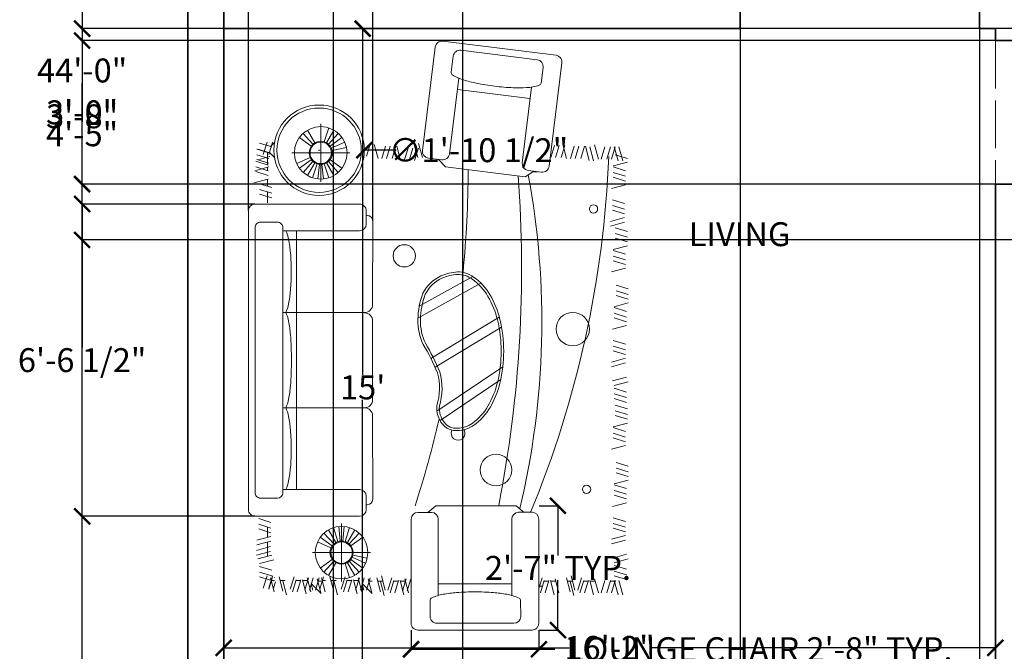
# Model space of a CAD drawing. Units: inches. Extents: x 43 to 543, y 36 to 629.
# Tile 2 of 5: x 43 to 290, y 189 to 348. Entities that reach past the tile are written whole.
import ezdxf

# ---------------------------------------------------------------- set-up
doc = ezdxf.new("R2010")
doc.units = ezdxf.units.IN
doc.header["$MEASUREMENT"] = 0
doc.linetypes.add('ACAD_ISO02W100', pattern=[15, 12, -3])
for name, color, linetype, lineweight in [('A-ANNO-DIMS', 2, 'Continuous', 18), ('A-AREA-IDEN', 7, 'Continuous', 25), ('A-FURN', 8, 'Continuous', 13), ('A-WALL', 7, 'Continuous', 35), ('A-WALL-OVHD', 7, 'ACAD_ISO02W100', 18)]:
    doc.layers.add(name, color=color, linetype=linetype, lineweight=lineweight)
doc.styles.get("Standard").update_dxf_attribs({"font": 'arial.ttf'})
doc.dimstyles.get("Standard").update_dxf_attribs({"dimtxt": 6, "dimasz": 4, "dimexe": 0.18, "dimexo": 0.0625, "dimgap": 0.09, "dimtad": 0, "dimtih": 1, "dimtoh": 1, "dimdec": 0, "dimzin": 0, "dimdsep": 46, "dimlunit": 4, "dimtxsty": 'Standard', "dimblk": 'ARCHTICK', "dimcen": 0.09, "dimadec": 0, "dimazin": 0, "dimtfac": 1, "dimtdec": 0, "dimtofl": 0, "dimtmove": 0, "dimatfit": 3, "dimldrblk": 'ARCHTICK', "dimfxl": 1, "dimtolj": 1, "dimtzin": 0, "dimarcsym": 1})

# ---------------------------------------------------------------- blocks, each defined once
blk = doc.blocks.new('_ArchTick')
at = {"color": 0, "linetype": 'ByBlock', "const_width": 0.15}
blk.add_lwpolyline([(-0.5, -0.5), (0.5, 0.5)], dxfattribs=at)
blk = doc.blocks.new('*D10')
at = {"layer": 'A-ANNO-DIMS', "color": 0, "lineweight": -2, "transparency": 16777216}
for p, q in [((93.88, 165.58), (93.88, 190.33)), ((93.88, 190.15), (180.51, 190.15)), ((287.38, 190.15), (200.74, 190.15)), ((287.38, 165.58), (287.38, 190.33))]:
    blk.add_line(p, q, dxfattribs=at)
at = {"layer": 'Defpoints', "color": 0, "transparency": 16777216}
for p in [(287.38, 190.15), (93.88, 165.52), (287.38, 165.52)]:
    blk.add_point(p, dxfattribs=at)
at = {"layer": 'A-ANNO-DIMS', "color": 0, "lineweight": -2, "transparency": 16777216, "xscale": 4, "yscale": 4, "zscale": 4, "rotation": 180}
blk.add_blockref('_ArchTick', (93.88, 190.15), dxfattribs=at)
at = {"layer": 'A-ANNO-DIMS', "color": 0, "lineweight": -2, "transparency": 16777216, "xscale": 4, "yscale": 4, "zscale": 4}
blk.add_blockref('_ArchTick', (287.38, 190.15), dxfattribs=at)
at = {"layer": 'A-ANNO-DIMS', "color": 0, "transparency": 16777216, "insert": (190.63, 190.15), "char_height": 6, "attachment_point": 5}
blk.add_mtext('\\A1;16\'-2"', dxfattribs=at)
blk = doc.blocks.new('*D11')
at = {"layer": 'A-ANNO-DIMS', "color": 0, "lineweight": -2, "transparency": 16777216}
for p, q in [((93.94, 345.52), (128.91, 345.52)), ((128.73, 345.52), (128.73, 258.67)), ((128.73, 165.52), (128.73, 252.36)), ((93.94, 165.52), (128.91, 165.52))]:
    blk.add_line(p, q, dxfattribs=at)
at = {"layer": 'Defpoints', "color": 0, "transparency": 16777216}
for p in [(93.88, 345.52), (128.73, 345.52), (93.88, 165.52)]:
    blk.add_point(p, dxfattribs=at)
at = {"layer": 'A-ANNO-DIMS', "color": 0, "lineweight": -2, "transparency": 16777216, "xscale": 4, "yscale": 4, "zscale": 4}
for p, rotation in [((128.73, 345.52), 90), ((128.73, 165.52), 270)]:
    blk.add_blockref('_ArchTick', p, dxfattribs=dict(at, rotation=rotation))
at = {"layer": 'A-ANNO-DIMS', "color": 0, "transparency": 16777216, "insert": (128.73, 255.52), "char_height": 6, "attachment_point": 5}
blk.add_mtext("\\A1;15'", dxfattribs=at)
blk = doc.blocks.new('CHAIR-LOUNGE')
for p, q in [((4.21, 29.53, -275.77), (6.22, 31.19, -275.77)), ((26.33, 31.2, -275.77), (6.22, 31.19, -275.77)), ((28.38, 29.51, -275.77), (26.33, 31.2, -275.77)), ((0, 27.82, -275.77), (0.01, 1.7, -275.77)), ((5.1, 29.53, -275.77), (1.7, 29.53, -275.77)), ((6.81, 8.69, -275.77), (6.8, 27.83, -275.77)), ((25.21, 8.69, -275.77), (25.21, 27.83, -275.77)), ((30.31, 29.54, -275.77), (26.91, 29.54, -275.77)), ((32.02, 1.71, -275.77), (32.01, 27.84, -275.77)), ((6.97, 11.58, -275.77), (25.09, 11.58, -275.77)), ((4.77, 3.4, -275.77), (4.77, 7.47, -275.77)), ((27.47, 3.41, -275.77), (27.46, 7.38, -275.77)), ((1.71, 0, -275.77), (30.32, 0.01, -275.77)), ((6.47, 1.7, -275.77), (25.77, 1.71, -275.77))]:
    blk.add_line(p, q)
for centre, radius, start, end in [((1.7, 27.82, -275.77), 1.7, 90.0228, 180.0228), ((5.1, 27.83, -275.77), 1.7, 0.0228, 90.0228), ((26.91, 27.83, -275.77), 1.7, 90.0228, 180.0228), ((30.31, 27.84, -275.77), 1.7, 0.0228, 90.0228), ((5.45, 7.47, -275.77), 0.68, 113.7374, 180.0228), ((10.4, -3.79, -275.77), 12.98, 100.5374, 113.7374), ((13.77, -21.88, -275.77), 31.38, 94.419, 100.5374), ((16.03, -51.17, -275.77), 60.76, 90.0228, 94.419), ((16.03, -51.17, -275.77), 60.76, 85.6266, 90.0228), ((18.27, -21.88, -275.77), 31.38, 79.5083, 85.6266), ((21.62, -3.79, -275.77), 12.98, 65.1817, 79.5083), ((26.78, 7.38, -275.77), 0.68, 0.0228, 65.1817), ((6.47, 3.4, -275.77), 1.7, 180.0228, 270.0228), ((25.77, 3.41, -275.77), 1.7, 270.0228, 0.0228), ((1.71, 1.7, -275.77), 1.7, 180.0228, 270.0228), ((30.32, 1.71, -275.77), 1.7, 270.0228, 0.0228)]:
    blk.add_arc(centre, radius, start, end)
blk = doc.blocks.new('*D29')
at = {"layer": 'A-ANNO-DIMS', "color": 0, "lineweight": -2, "transparency": 16777216}
for p, q in [((140.89, 194.57), (140.89, 189.65)), ((172.91, 194.57), (172.91, 189.65)), ((140.89, 189.83), (172.91, 189.83)), ((172.91, 189.83), (176.91, 189.83))]:
    blk.add_line(p, q, dxfattribs=at)
at = {"layer": 'Defpoints', "color": 0, "transparency": 16777216}
for p in [(140.89, 194.63), (172.91, 194.63), (172.91, 189.83)]:
    blk.add_point(p, dxfattribs=at)
at = {"layer": 'A-ANNO-DIMS', "color": 0, "lineweight": -2, "transparency": 16777216, "xscale": 4, "yscale": 4, "zscale": 4, "rotation": 180}
blk.add_blockref('_ArchTick', (140.89, 189.83), dxfattribs=at)
at = {"layer": 'A-ANNO-DIMS', "color": 0, "lineweight": -2, "transparency": 16777216, "xscale": 4, "yscale": 4, "zscale": 4}
blk.add_blockref('_ArchTick', (172.91, 189.83), dxfattribs=at)
at = {"layer": 'A-ANNO-DIMS', "color": 0, "transparency": 16777216, "insert": (228.22, 189.83), "char_height": 6, "attachment_point": 5}
blk.add_mtext('\\A1;LOUNGE CHAIR 2\'-8" TYP.', dxfattribs=at)
blk = doc.blocks.new('*D30')
at = {"layer": 'A-ANNO-DIMS', "color": 0, "lineweight": -2, "transparency": 16777216}
for p, q in [((172.97, 225.83), (177.89, 225.83)), ((177.71, 225.83), (177.71, 213.34)), ((177.71, 194.63), (177.71, 207.13)), ((172.97, 194.63), (177.89, 194.63))]:
    blk.add_line(p, q, dxfattribs=at)
at = {"layer": 'Defpoints', "color": 0, "transparency": 16777216}
for p in [(172.91, 225.83), (177.71, 225.83), (172.91, 194.63)]:
    blk.add_point(p, dxfattribs=at)
at = {"layer": 'A-ANNO-DIMS', "color": 0, "lineweight": -2, "transparency": 16777216, "xscale": 4, "yscale": 4, "zscale": 4}
for p, rotation in [((177.71, 225.83), 90), ((177.71, 194.63), 270)]:
    blk.add_blockref('_ArchTick', p, dxfattribs=dict(at, rotation=rotation))
at = {"layer": 'A-ANNO-DIMS', "color": 0, "transparency": 16777216, "insert": (177.71, 210.23), "char_height": 6, "attachment_point": 5}
blk.add_mtext('\\A1;2\'-7" TYP.', dxfattribs=at)
blk = doc.blocks.new('*D38')
at = {"layer": 'A-ANNO-DIMS', "color": 0, "lineweight": -2, "transparency": 16777216}
for p, q in [((84.82, 599.02), (58.2, 599.02)), ((58.38, 599.02), (58.38, 338.17)), ((58.38, 71.02), (58.38, 331.86)), ((84.82, 71.02), (58.2, 71.02))]:
    blk.add_line(p, q, dxfattribs=at)
at = {"layer": 'Defpoints', "color": 0, "transparency": 16777216}
for p in [(58.38, 599.02), (84.88, 599.02), (84.88, 71.02)]:
    blk.add_point(p, dxfattribs=at)
at = {"layer": 'A-ANNO-DIMS', "color": 0, "lineweight": -2, "transparency": 16777216, "xscale": 4, "yscale": 4, "zscale": 4}
for p, rotation in [((58.38, 599.02), 90), ((58.38, 71.02), 270)]:
    blk.add_blockref('_ArchTick', p, dxfattribs=dict(at, rotation=rotation))
at = {"layer": 'A-ANNO-DIMS', "color": 0, "transparency": 16777216, "insert": (58.38, 335.02), "char_height": 6, "attachment_point": 5}
blk.add_mtext('\\A1;44\'-0"', dxfattribs=at)
blk = doc.blocks.new('*D44')
at = {"layer": 'A-ANNO-DIMS', "color": 0, "lineweight": -2, "transparency": 16777216}
for p, q in [((121.33, 384.5), (121.33, 44.34)), ((153.74, 384.5), (153.74, 44.34)), ((121.33, 44.52), (122.43, 44.52)), ((153.74, 44.52), (152.64, 44.52))]:
    blk.add_line(p, q, dxfattribs=at)
at = {"layer": 'Defpoints', "color": 0, "transparency": 16777216}
for p in [(121.33, 384.57), (153.74, 384.57), (153.74, 44.52)]:
    blk.add_point(p, dxfattribs=at)
at = {"layer": 'A-ANNO-DIMS', "color": 0, "lineweight": -2, "transparency": 16777216, "xscale": 4, "yscale": 4, "zscale": 4, "rotation": 180}
blk.add_blockref('_ArchTick', (121.33, 44.52), dxfattribs=at)
at = {"layer": 'A-ANNO-DIMS', "color": 0, "lineweight": -2, "transparency": 16777216, "xscale": 4, "yscale": 4, "zscale": 4}
blk.add_blockref('_ArchTick', (153.74, 44.52), dxfattribs=at)
at = {"layer": 'A-ANNO-DIMS', "color": 0, "transparency": 16777216, "insert": (137.54, 44.52), "char_height": 6, "attachment_point": 5}
blk.add_mtext('\\A1;2\'-8 1/2"', dxfattribs=at)
blk = doc.blocks.new('*D49')
at = {"layer": 'A-ANNO-DIMS', "color": 0, "lineweight": -2, "transparency": 16777216}
for p, q in [((371.32, 345.52), (58.2, 345.52)), ((58.38, 345.52), (58.38, 322.16)), ((58.38, 292.52), (58.38, 315.88)), ((371.32, 292.52), (58.2, 292.52))]:
    blk.add_line(p, q, dxfattribs=at)
at = {"layer": 'Defpoints', "color": 0, "transparency": 16777216}
for p in [(58.38, 345.52), (371.38, 345.52), (371.38, 292.52)]:
    blk.add_point(p, dxfattribs=at)
at = {"layer": 'A-ANNO-DIMS', "color": 0, "lineweight": -2, "transparency": 16777216, "xscale": 4, "yscale": 4, "zscale": 4}
for p, rotation in [((58.38, 345.52), 90), ((58.38, 292.52), 270)]:
    blk.add_blockref('_ArchTick', p, dxfattribs=dict(at, rotation=rotation))
at = {"layer": 'A-ANNO-DIMS', "color": 0, "transparency": 16777216, "insert": (58.38, 319.02), "char_height": 6, "attachment_point": 5}
blk.add_mtext('\\A1;4\'-5"', dxfattribs=at)
blk = doc.blocks.new('*D54')
at = {"layer": 'A-ANNO-DIMS', "color": 0, "lineweight": -2, "transparency": 16777216}
for p, q in [((223.38, 345.45), (223.38, 44.34)), ((283.38, 345.45), (283.38, 44.34)), ((223.38, 44.52), (245.31, 44.52)), ((283.38, 44.52), (261.44, 44.52))]:
    blk.add_line(p, q, dxfattribs=at)
at = {"layer": 'Defpoints', "color": 0, "transparency": 16777216}
for p in [(223.38, 345.52), (283.38, 345.52), (283.38, 44.52)]:
    blk.add_point(p, dxfattribs=at)
at = {"layer": 'A-ANNO-DIMS', "color": 0, "lineweight": -2, "transparency": 16777216, "xscale": 4, "yscale": 4, "zscale": 4, "rotation": 180}
blk.add_blockref('_ArchTick', (223.38, 44.52), dxfattribs=at)
at = {"layer": 'A-ANNO-DIMS', "color": 0, "lineweight": -2, "transparency": 16777216, "xscale": 4, "yscale": 4, "zscale": 4}
blk.add_blockref('_ArchTick', (283.38, 44.52), dxfattribs=at)
at = {"layer": 'A-ANNO-DIMS', "color": 0, "transparency": 16777216, "insert": (253.38, 44.52), "char_height": 6, "attachment_point": 5}
blk.add_mtext('\\A1;5\'-0"', dxfattribs=at)
blk = doc.blocks.new('*D55')
at = {"layer": 'A-ANNO-DIMS', "color": 0, "lineweight": -2, "transparency": 16777216}
for p, q in [((287.32, 342.52), (58.2, 342.52)), ((58.38, 342.52), (58.38, 327.67)), ((58.38, 306.52), (58.38, 321.36)), ((287.32, 306.52), (58.2, 306.52))]:
    blk.add_line(p, q, dxfattribs=at)
at = {"layer": 'Defpoints', "color": 0, "transparency": 16777216}
for p in [(58.38, 342.52), (287.38, 342.52), (287.38, 306.52)]:
    blk.add_point(p, dxfattribs=at)
at = {"layer": 'A-ANNO-DIMS', "color": 0, "lineweight": -2, "transparency": 16777216, "xscale": 4, "yscale": 4, "zscale": 4}
for p, rotation in [((58.38, 342.52), 90), ((58.38, 306.52), 270)]:
    blk.add_blockref('_ArchTick', p, dxfattribs=dict(at, rotation=rotation))
at = {"layer": 'A-ANNO-DIMS', "color": 0, "transparency": 16777216, "insert": (58.38, 324.52), "char_height": 6, "attachment_point": 5}
blk.add_mtext('\\A1;3\'-0"', dxfattribs=at)
blk = doc.blocks.new('*D56')
at = {"layer": 'A-ANNO-DIMS', "color": 0, "lineweight": -2, "transparency": 16777216}
for p, q in [((101.72, 301.52), (58.2, 301.52)), ((58.38, 301.52), (58.38, 265.54)), ((58.38, 223.17), (58.38, 259.15)), ((101.72, 223.17), (58.2, 223.17))]:
    blk.add_line(p, q, dxfattribs=at)
at = {"layer": 'Defpoints', "color": 0, "transparency": 16777216}
for p in [(58.38, 301.52), (101.78, 301.52), (101.78, 223.17)]:
    blk.add_point(p, dxfattribs=at)
at = {"layer": 'A-ANNO-DIMS', "color": 0, "lineweight": -2, "transparency": 16777216, "xscale": 4, "yscale": 4, "zscale": 4}
for p, rotation in [((58.38, 301.52), 90), ((58.38, 223.17), 270)]:
    blk.add_blockref('_ArchTick', p, dxfattribs=dict(at, rotation=rotation))
at = {"layer": 'A-ANNO-DIMS', "color": 0, "transparency": 16777216, "insert": (58.38, 262.35), "char_height": 6, "attachment_point": 5}
blk.add_mtext('\\A1;6\'-6 1/2"', dxfattribs=at)
blk = doc.blocks.new('*D57')
at = {"layer": 'A-ANNO-DIMS', "color": 0, "lineweight": -2, "transparency": 16777216}
for p, q in [((100.07, 299.91), (100.07, 625.7)), ((100.07, 625.52), (107.55, 625.52)), ((131.25, 625.52), (123.78, 625.52)), ((131.25, 297.32), (131.25, 625.7))]:
    blk.add_line(p, q, dxfattribs=at)
at = {"layer": 'Defpoints', "color": 0, "transparency": 16777216}
for p in [(131.25, 625.52), (100.07, 299.85), (131.25, 297.26)]:
    blk.add_point(p, dxfattribs=at)
at = {"layer": 'A-ANNO-DIMS', "color": 0, "lineweight": -2, "transparency": 16777216, "xscale": 4, "yscale": 4, "zscale": 4, "rotation": 180}
blk.add_blockref('_ArchTick', (100.07, 625.52), dxfattribs=at)
at = {"layer": 'A-ANNO-DIMS', "color": 0, "lineweight": -2, "transparency": 16777216, "xscale": 4, "yscale": 4, "zscale": 4}
blk.add_blockref('_ArchTick', (131.25, 625.52), dxfattribs=at)
at = {"layer": 'A-ANNO-DIMS', "color": 0, "transparency": 16777216, "insert": (115.66, 625.52), "char_height": 6, "attachment_point": 5}
blk.add_mtext('\\A1;2\'-7"', dxfattribs=at)
blk = doc.blocks.new('*D58')
at = {"layer": 'A-ANNO-DIMS', "color": 0, "lineweight": -2, "transparency": 16777216}
for p, q in [((93.88, 345.58), (93.88, 625.7)), ((93.88, 625.52), (100.07, 625.52)), ((100.07, 299.91), (100.07, 625.7)), ((100.07, 625.52), (104.07, 625.52))]:
    blk.add_line(p, q, dxfattribs=at)
at = {"layer": 'Defpoints', "color": 0, "transparency": 16777216}
for p in [(100.07, 625.52), (93.88, 345.52), (100.07, 299.85)]:
    blk.add_point(p, dxfattribs=at)
at = {"layer": 'A-ANNO-DIMS', "color": 0, "lineweight": -2, "transparency": 16777216, "xscale": 4, "yscale": 4, "zscale": 4, "rotation": 180}
blk.add_blockref('_ArchTick', (93.88, 625.52), dxfattribs=at)
at = {"layer": 'A-ANNO-DIMS', "color": 0, "lineweight": -2, "transparency": 16777216, "xscale": 4, "yscale": 4, "zscale": 4}
blk.add_blockref('_ArchTick', (100.07, 625.52), dxfattribs=at)
at = {"layer": 'A-ANNO-DIMS', "color": 0, "transparency": 16777216, "insert": (112.13, 625.52), "char_height": 6, "attachment_point": 5}
blk.add_mtext('\\A1;0\'-6"', dxfattribs=at)
blk = doc.blocks.new('*D59')
at = {"layer": 'A-ANNO-DIMS', "color": 0, "lineweight": -2, "transparency": 16777216}
for p, q in [((93.82, 345.52), (58.2, 345.52)), ((58.38, 345.52), (58.38, 326.67)), ((58.38, 301.52), (58.38, 320.36)), ((101.72, 301.52), (58.2, 301.52))]:
    blk.add_line(p, q, dxfattribs=at)
at = {"layer": 'Defpoints', "color": 0, "transparency": 16777216}
for p in [(93.88, 345.52), (58.38, 301.52), (101.78, 301.52)]:
    blk.add_point(p, dxfattribs=at)
at = {"layer": 'A-ANNO-DIMS', "color": 0, "lineweight": -2, "transparency": 16777216, "xscale": 4, "yscale": 4, "zscale": 4}
for p, rotation in [((58.38, 345.52), 90), ((58.38, 301.52), 270)]:
    blk.add_blockref('_ArchTick', p, dxfattribs=dict(at, rotation=rotation))
at = {"layer": 'A-ANNO-DIMS', "color": 0, "transparency": 16777216, "insert": (58.38, 323.52), "char_height": 6, "attachment_point": 5}
blk.add_mtext('\\A1;3\'-8"', dxfattribs=at)
blk = doc.blocks.new('*D60')
at = {"layer": 'A-ANNO-DIMS', "color": 0, "lineweight": -2, "transparency": 16777216}
for p, q in [((121.33, 384.5), (121.33, 44.34)), ((93.88, 349.95), (93.88, 44.34)), ((93.88, 44.52), (121.33, 44.52)), ((121.33, 44.52), (125.33, 44.52))]:
    blk.add_line(p, q, dxfattribs=at)
at = {"layer": 'Defpoints', "color": 0, "transparency": 16777216}
for p in [(121.33, 384.57), (93.88, 350.02), (121.33, 44.52)]:
    blk.add_point(p, dxfattribs=at)
at = {"layer": 'A-ANNO-DIMS', "color": 0, "lineweight": -2, "transparency": 16777216, "xscale": 4, "yscale": 4, "zscale": 4, "rotation": 180}
blk.add_blockref('_ArchTick', (93.88, 44.52), dxfattribs=at)
at = {"layer": 'A-ANNO-DIMS', "color": 0, "lineweight": -2, "transparency": 16777216, "xscale": 4, "yscale": 4, "zscale": 4}
blk.add_blockref('_ArchTick', (121.33, 44.52), dxfattribs=at)
at = {"layer": 'A-ANNO-DIMS', "color": 0, "transparency": 16777216, "insert": (140.43, 44.52), "char_height": 6, "attachment_point": 5}
blk.add_mtext('\\A1;2\'-3 1/2"', dxfattribs=at)
blk = doc.blocks.new('*D67')
at = {"layer": 'A-ANNO-DIMS', "color": 0, "lineweight": -2, "transparency": 16777216}
for p, q in [((287.38, 306.45), (287.38, 44.34)), ((291.88, 306.45), (291.88, 44.34)), ((287.38, 44.52), (291.88, 44.52)), ((291.88, 44.52), (295.88, 44.52))]:
    blk.add_line(p, q, dxfattribs=at)
at = {"layer": 'Defpoints', "color": 0, "transparency": 16777216}
for p in [(287.38, 306.52), (291.88, 306.52), (291.88, 44.52)]:
    blk.add_point(p, dxfattribs=at)
at = {"layer": 'A-ANNO-DIMS', "color": 0, "lineweight": -2, "transparency": 16777216, "xscale": 4, "yscale": 4, "zscale": 4, "rotation": 180}
blk.add_blockref('_ArchTick', (287.38, 44.52), dxfattribs=at)
at = {"layer": 'A-ANNO-DIMS', "color": 0, "lineweight": -2, "transparency": 16777216, "xscale": 4, "yscale": 4, "zscale": 4}
blk.add_blockref('_ArchTick', (291.88, 44.52), dxfattribs=at)
at = {"layer": 'A-ANNO-DIMS', "color": 0, "transparency": 16777216, "insert": (310.93, 44.52), "char_height": 6, "attachment_point": 5}
blk.add_mtext('\\A1;0\'-4 1/2"', dxfattribs=at)
blk = doc.blocks.new('*D68')
at = {"layer": 'A-ANNO-DIMS', "color": 0, "lineweight": -2, "transparency": 16777216}
for p, q in [((117.72, 315.02), (117.9, 315.02)), ((117.81, 314.93), (117.81, 315.11)), ((137.15, 315.02), (129.15, 315.02))]:
    blk.add_line(p, q, dxfattribs=at)
at = {"layer": 'Defpoints', "color": 0, "transparency": 16777216}
for p in [(106.47, 315.02), (129.15, 315.02)]:
    blk.add_point(p, dxfattribs=at)
at = {"layer": 'A-ANNO-DIMS', "color": 0, "lineweight": -2, "transparency": 16777216, "xscale": 4, "yscale": 4, "zscale": 4, "rotation": 179.9982316117439}
blk.add_blockref('_ArchTick', (129.15, 315.02), dxfattribs=at)
at = {"layer": 'A-ANNO-DIMS', "color": 0, "transparency": 16777216, "insert": (157.8, 315.02), "char_height": 6, "attachment_point": 5}
blk.add_mtext('\\A1;∅1\'-10 1/2"', dxfattribs=at)

msp = doc.modelspace()

# ---------------------------------------------------------------- linework, layer by layer
at = {"layer": 'A-FURN'}
for p, q in [((118.22, 314.35, -275.77), (118.22, 321.62, -275.77)), ((116.27, 316.52, -275.77), (113.81, 319.25, -275.77)), ((116.76, 316.88, -275.77), (114.92, 320.06, -275.77)), ((119.11, 317.12, -275.77), (120.25, 320.62, -275.77)), ((119.67, 316.88, -275.77), (121.51, 320.06, -275.77)), ((120.16, 316.52, -275.77), (122.62, 319.25, -275.77)), ((105.95, 315.88, -275.77), (102.89, 316.82, -275.77)), ((104.75, 317.04, -275.77), (103.81, 313.98, -275.77)), ((106.16, 317.04, -275.77), (105.22, 313.98, -275.77)), ((105.66, 315.97, -275.77), (106.63, 316.94, -275.77)), ((115.86, 316.07, -275.77), (112.89, 318.23, -275.77)), ((120.57, 316.07, -275.77), (123.55, 318.23, -275.77)), ((120.87, 315.54, -275.77), (124.23, 317.03, -275.77)), ((130.63, 316.57, -275.77), (129.69, 313.51, -275.77)), ((132.59, 312.95, -275.77), (131.65, 316.47, -275.77)), ((142.54, 313.18, -275.77), (141.6, 316.71, -275.77)), ((143.71, 313.18, -275.77), (142.77, 316.71, -275.77)), ((175.93, 313.18, -275.77), (176.87, 316.24, -275.77)), ((177.1, 313.18, -275.77), (178.04, 316.24, -275.77)), ((178.52, 313.18, -275.77), (179.46, 316.24, -275.77)), ((179.87, 312.95, -275.77), (178.93, 316.47, -275.77)), ((186.88, 316.33, -275.77), (187.83, 312.8, -275.77)), ((105.24, 314.35, -275.77), (102.19, 315.29, -275.77)), ((105.24, 312.94, -275.77), (102.19, 313.88, -275.77)), ((105.48, 314.35, -275.77), (102.42, 315.29, -275.77)), ((104.85, 311.34, -275.77), (104.85, 314.55, -275.77)), ((106.63, 313.15, -275.77), (105.36, 314.42, -275.77)), ((118.22, 314.35, -275.77), (110.95, 314.35, -275.77)), ((115.57, 314.82, -275.77), (115.38, 315.01, -275.77)), ((118.22, 314.35, -275.77), (118.22, 307.09, -275.77)), ((118.22, 314.35, -275.77), (125.48, 314.35, -275.77)), ((121.06, 314.96, -275.77), (124.66, 315.72, -275.77)), ((133.53, 312.95, -275.77), (134.48, 316, -275.77)), ((134.71, 312.95, -275.77), (135.65, 316, -275.77)), ((136.12, 312.95, -275.77), (137.06, 316, -275.77)), ((138.24, 312.47, -275.77), (137.3, 316, -275.77)), ((139.18, 312.47, -275.77), (140.12, 315.53, -275.77)), ((140.36, 312.47, -275.77), (141.3, 315.53, -275.77)), ((141.77, 312.47, -275.77), (142.71, 315.53, -275.77)), ((180.82, 312.95, -275.77), (181.76, 316, -275.77)), ((181.99, 312.95, -275.77), (182.93, 316, -275.77)), ((183.4, 312.95, -275.77), (184.35, 316, -275.77)), ((185.52, 312.47, -275.77), (184.58, 316, -275.77)), ((185.71, 315.86, -275.77), (186.65, 312.33, -275.77)), ((189.47, 315.86, -275.77), (188.53, 312.8, -275.77)), ((190.88, 315.86, -275.77), (189.94, 312.8, -275.77)), ((192.06, 315.86, -275.77), (191.12, 312.8, -275.77)), ((191.82, 315.86, -275.77), (192.76, 312.33, -275.77)), ((195.1, 312.94, -275.77), (192.05, 313.88, -275.77)), ((193, 315.86, -275.77), (193.94, 312.33, -275.77)), ((105.01, 311.29, -275.77), (101.95, 312.23, -275.77)), ((105.24, 311.76, -275.77), (102.19, 312.71, -275.77)), ((105.48, 313.41, -275.77), (102.49, 312.61, -275.77)), ((115.56, 313.17, -275.77), (112.2, 311.67, -275.77)), ((115.86, 312.64, -275.77), (112.89, 310.48, -275.77)), ((116.27, 312.19, -275.77), (113.81, 309.46, -275.77)), ((116.76, 311.83, -275.77), (114.92, 308.65, -275.77)), ((117.32, 311.59, -275.77), (116.18, 308.09, -275.77)), ((117.91, 311.46, -275.77), (117.53, 307.8, -275.77)), ((118.52, 311.46, -275.77), (118.9, 307.8, -275.77)), ((118.87, 311.52, -275.77), (118.68, 311.71, -275.77)), ((119.11, 311.59, -275.77), (120.25, 308.09, -275.77)), ((119.67, 311.83, -275.77), (121.51, 308.65, -275.77)), ((120.16, 312.19, -275.77), (122.62, 309.46, -275.77)), ((120.57, 312.64, -275.77), (123.55, 310.48, -275.77)), ((195.1, 312, -275.77), (191.58, 311.06, -275.77)), ((105.24, 310.82, -275.77), (101.72, 309.88, -275.77)), ((105.01, 309.88, -275.77), (101.95, 310.82, -275.77)), ((105.01, 308.7, -275.77), (101.95, 309.65, -275.77)), ((104.85, 309.93, -275.77), (104.85, 310.72, -275.77)), ((171.43, 309.63, -275.77), (172.74, 309.63, -275.77)), ((194.63, 309.88, -275.77), (191.58, 310.82, -275.77)), ((194.63, 308.47, -275.77), (191.58, 309.41, -275.77)), ((105.01, 307.76, -275.77), (101.48, 306.82, -275.77)), ((105.95, 305.65, -275.77), (102.89, 306.59, -275.77)), ((104.85, 305.99, -275.77), (104.85, 307.72, -275.77)), ((194.63, 306.35, -275.77), (191.11, 305.41, -275.77)), ((194.63, 307.29, -275.77), (191.58, 308.23, -275.77)), ((105.95, 304.23, -275.77), (102.89, 305.18, -275.77)), ((105.95, 303.06, -275.77), (102.89, 304, -275.77)), ((104.85, 301.82, -275.77), (104.85, 304.57, -275.77)), ((101.78, 301.52, -275.77), (127.93, 301.51, -275.77)), ((194.4, 301.65, -275.77), (191.34, 302.59, -275.77)), ((100.07, 299.85, -275.77), (100.08, 224.87, -275.77)), ((129.62, 298.75, -275.77), (129.62, 296.49, -275.77)), ((129.63, 298.58, -275.77), (129.63, 299.81, -275.77)), ((194.4, 300.23, -275.77), (191.34, 301.17, -275.77)), ((194.4, 299.06, -275.77), (191.34, 300, -275.77)), ((103.14, 296.97, -275.77), (107.36, 296.96, -275.77)), ((129.63, 298.62, -275.77), (129.89, 298.62, -275.77)), ((131.24, 276.33, -275.77), (131.25, 297.26, -275.77)), ((194.4, 298.12, -275.77), (190.87, 297.17, -275.77)), ((194.4, 296.94, -275.77), (190.87, 296, -275.77)), ((101.75, 295.61, -275.77), (101.78, 229.09, -275.77)), ((108.71, 274.29, -275.77), (108.72, 295.6, -275.77)), ((108.72, 294.8, -275.77), (127.92, 294.79, -275.77)), ((112.11, 274.29, -275.77), (112.12, 294.8, -275.77)), ((195.1, 294.59, -275.77), (192.05, 295.53, -275.77)), ((195.1, 293.17, -275.77), (192.05, 294.12, -275.77)), ((195.1, 292, -275.77), (192.05, 292.94, -275.77)), ((195.1, 291.06, -275.77), (191.58, 290.12, -275.77)), ((194.63, 288.94, -275.77), (191.58, 289.88, -275.77)), ((194.63, 287.53, -275.77), (191.58, 288.47, -275.77)), ((194.63, 286.35, -275.77), (191.58, 287.29, -275.77)), ((194.63, 285.41, -275.77), (191.11, 284.47, -275.77)), ((142.6, 272.9, -275.77), (158.38, 281.63, -275.77)), ((142.93, 275.91, -275.77), (156.35, 283.34, -275.77)), ((195.34, 280.23, -275.77), (192.28, 281.17, -275.77)), ((195.34, 278.82, -275.77), (192.28, 279.76, -275.77)), ((195.34, 276.7, -275.77), (191.81, 275.76, -275.77)), ((195.34, 277.64, -275.77), (192.28, 278.58, -275.77)), ((108.71, 274.3, -275.77), (108.72, 229.09, -275.77)), ((108.71, 274.3, -275.77), (123.9, 274.29, -275.77)), ((112.11, 274.3, -275.77), (112.12, 229.89, -275.77)), ((123.9, 274.29, -275.77), (129.2, 274.29, -275.77)), ((194.87, 274.58, -275.77), (191.81, 275.53, -275.77)), ((194.87, 273.17, -275.77), (191.81, 274.11, -275.77)), ((131.24, 252.44, -275.77), (131.24, 272.25, -275.77)), ((145.83, 262.8, -275.77), (163, 273.13, -275.77)), ((194.87, 272, -275.77), (191.81, 272.94, -275.77)), ((146.91, 260.62, -275.77), (163.55, 270.63, -275.77)), ((194.87, 271.05, -275.77), (191.34, 270.11, -275.77)), ((194.63, 266.35, -275.77), (191.58, 267.29, -275.77)), ((194.63, 264.94, -275.77), (191.58, 265.88, -275.77)), ((194.63, 263.76, -275.77), (191.58, 264.7, -275.77)), ((194.63, 262.82, -275.77), (191.11, 261.88, -275.77)), ((147.37, 249.53, -275.77), (163.87, 260.68, -275.77)), ((194.63, 261.64, -275.77), (191.11, 260.7, -275.77)), ((148.13, 247.21, -275.77), (163.36, 257.5, -275.77)), ((194.87, 258.11, -275.77), (191.34, 257.17, -275.77)), ((195.34, 256.94, -275.77), (191.81, 255.99, -275.77)), ((194.87, 254.35, -275.77), (191.81, 255.29, -275.77)), ((194.87, 252.94, -275.77), (191.81, 253.88, -275.77)), ((194.87, 251.76, -275.77), (191.81, 252.7, -275.77)), ((108.71, 250.39, -275.77), (123.9, 250.4, -275.77)), ((123.9, 250.4, -275.77), (129.2, 250.4, -275.77)), ((195.1, 250.11, -275.77), (192.05, 251.05, -275.77)), ((195.1, 248.7, -275.77), (192.05, 249.64, -275.77)), ((131.24, 248.36, -275.77), (131.25, 227.43, -275.77)), ((195.1, 247.52, -275.77), (192.05, 248.46, -275.77)), ((195.1, 246.58, -275.77), (191.58, 245.64, -275.77)), ((194.63, 244.46, -275.77), (191.58, 245.41, -275.77)), ((194.63, 243.05, -275.77), (191.58, 243.99, -275.77)), ((194.63, 241.88, -275.77), (191.58, 242.82, -275.77)), ((194.63, 240.94, -275.77), (191.11, 239.99, -275.77)), ((195.34, 235.76, -275.77), (192.28, 236.7, -275.77)), ((195.34, 234.35, -275.77), (192.28, 235.29, -275.77)), ((195.34, 232.23, -275.77), (191.81, 231.29, -275.77)), ((195.34, 233.17, -275.77), (192.28, 234.11, -275.77)), ((108.72, 229.89, -275.77), (127.92, 229.9, -275.77)), ((194.87, 230.11, -275.77), (191.81, 231.05, -275.77)), ((194.87, 228.7, -275.77), (191.81, 229.64, -275.77)), ((103.14, 227.73, -275.77), (107.36, 227.73, -275.77)), ((129.62, 225.95, -275.77), (129.62, 228.2, -275.77)), ((194.87, 227.52, -275.77), (191.81, 228.46, -275.77)), ((129.63, 226.11, -275.77), (129.63, 224.88, -275.77)), ((129.63, 226.07, -275.77), (129.89, 226.07, -275.77)), ((194.87, 226.58, -275.77), (191.34, 225.64, -275.77)), ((101.78, 223.17, -275.77), (127.93, 223.18, -275.77)), ((105.71, 221.64, -275.77), (102.66, 222.58, -275.77)), ((194.63, 221.87, -275.77), (191.58, 222.82, -275.77)), ((105.71, 220.23, -275.77), (102.66, 221.17, -275.77)), ((105.71, 219.05, -275.77), (102.66, 219.99, -275.77)), ((104.85, 217.88, -275.77), (104.85, 220.49, -275.77)), ((121.98, 216.58, -275.77), (120.14, 219.77, -275.77)), ((122.54, 216.83, -275.77), (121.4, 220.33, -275.77)), ((123.13, 216.96, -275.77), (122.75, 220.61, -275.77)), ((123.44, 221.38, -275.77), (123.44, 206.79, -275.77)), ((123.74, 216.96, -275.77), (124.12, 220.61, -275.77)), ((124.34, 216.83, -275.77), (125.47, 220.33, -275.77)), ((124.89, 216.58, -275.77), (126.73, 219.77, -275.77)), ((194.63, 220.46, -275.77), (191.58, 221.4, -275.77)), ((194.63, 219.29, -275.77), (191.58, 220.23, -275.77)), ((105.71, 218.11, -275.77), (102.19, 217.17, -275.77)), ((121.08, 215.77, -275.77), (118.11, 217.94, -275.77)), ((121.49, 216.23, -275.77), (119.03, 218.96, -275.77)), ((125.38, 216.23, -275.77), (127.84, 218.96, -275.77)), ((125.79, 215.77, -275.77), (128.77, 217.94, -275.77)), ((194.63, 218.35, -275.77), (191.11, 217.4, -275.77)), ((105.61, 215.56, -275.77), (102.08, 214.61, -275.77)), ((105.71, 216.93, -275.77), (102.19, 215.99, -275.77)), ((104.85, 213.11, -275.77), (104.85, 216.7, -275.77)), ((120.78, 215.25, -275.77), (117.42, 216.74, -275.77)), ((194.63, 217.17, -275.77), (191.11, 216.23, -275.77)), ((105.61, 214.38, -275.77), (102.08, 213.44, -275.77)), ((105.95, 213.4, -275.77), (102.42, 212.46, -275.77)), ((123.44, 214.06, -275.77), (116.17, 214.06, -275.77)), ((121.08, 212.35, -275.77), (118.11, 210.19, -275.77)), ((123.44, 214.06, -275.77), (130.7, 214.06, -275.77)), ((125.79, 212.35, -275.77), (128.77, 210.19, -275.77)), ((126.09, 212.88, -275.77), (129.45, 211.38, -275.77)), ((126.28, 213.46, -275.77), (129.88, 212.69, -275.77)), ((194.87, 213.64, -275.77), (191.34, 212.7, -275.77)), ((195.34, 212.46, -275.77), (191.81, 211.52, -275.77)), ((106.42, 212.23, -275.77), (102.89, 211.29, -275.77)), ((105.95, 209.64, -275.77), (102.89, 210.58, -275.77)), ((121.49, 211.9, -275.77), (119.03, 209.17, -275.77)), ((121.98, 211.54, -275.77), (120.14, 208.36, -275.77)), ((124.34, 211.29, -275.77), (125.47, 207.8, -275.77)), ((124.89, 211.54, -275.77), (126.73, 208.36, -275.77)), ((125.38, 211.9, -275.77), (127.84, 209.17, -275.77)), ((194.87, 209.87, -275.77), (191.81, 210.82, -275.77)), ((105.95, 208.23, -275.77), (102.89, 209.17, -275.77)), ((105.95, 207.05, -275.77), (102.89, 207.99, -275.77)), ((104.75, 208.21, -275.77), (103.81, 205.15, -275.77)), ((106.14, 207.95, -275.77), (105.2, 204.9, -275.77)), ((106.16, 208.21, -275.77), (105.22, 205.15, -275.77)), ((105.63, 207.72, -275.77), (106.57, 204.19, -275.77)), ((107.76, 207.95, -275.77), (108.7, 204.42, -275.77)), ((111.53, 207.95, -275.77), (110.59, 204.9, -275.77)), ((115.14, 207.72, -275.77), (114.19, 204.66, -275.77)), ((114.81, 207.72, -275.77), (115.75, 204.19, -275.77)), ((116.31, 207.72, -275.77), (115.37, 204.66, -275.77)), ((117.86, 207.74, -275.77), (116.92, 204.68, -275.77)), ((117.34, 207.5, -275.77), (118.28, 203.98, -275.77)), ((118.92, 207.95, -275.77), (117.98, 204.9, -275.77)), ((118.4, 207.72, -275.77), (119.35, 204.19, -275.77)), ((120.54, 207.95, -275.77), (121.48, 204.42, -275.77)), ((124.31, 207.95, -275.77), (123.36, 204.9, -275.77)), ((127.91, 207.72, -275.77), (126.97, 204.66, -275.77)), ((127.58, 207.72, -275.77), (128.53, 204.19, -275.77)), ((129.09, 207.72, -275.77), (128.15, 204.66, -275.77)), ((130.63, 207.74, -275.77), (129.69, 204.68, -275.77)), ((130.12, 207.5, -275.77), (131.06, 203.98, -275.77)), ((132.25, 207.74, -275.77), (133.19, 204.21, -275.77)), ((133.43, 208.21, -275.77), (134.37, 204.68, -275.77)), ((136.02, 207.74, -275.77), (135.08, 204.68, -275.77)), ((139.62, 207.5, -275.77), (138.68, 204.45, -275.77)), ((139.3, 207.5, -275.77), (140.24, 203.98, -275.77)), ((140.8, 207.5, -275.77), (139.86, 204.45, -275.77)), ((173.71, 207.74, -275.77), (172.9, 205.1, -275.77)), ((176.99, 207.5, -275.77), (177.93, 203.98, -275.77)), ((179.84, 207.74, -275.77), (180.78, 204.21, -275.77)), ((181.02, 208.21, -275.77), (181.96, 204.68, -275.77)), ((183.61, 207.74, -275.77), (182.66, 204.68, -275.77)), ((186.88, 207.5, -275.77), (187.83, 203.98, -275.77)), ((194.87, 208.46, -275.77), (191.81, 209.4, -275.77)), ((194.87, 207.29, -275.77), (191.81, 208.23, -275.77)), ((106.62, 207.08, -275.77), (105.88, 207.08, -275.77)), ((106.87, 206.69, -275.77), (106.4, 205.15, -275.77)), ((109.3, 207.08, -275.77), (108, 207.08, -275.77)), ((108.69, 207.01, -275.77), (109.63, 203.48, -275.77)), ((112.08, 207.25, -275.77), (111.14, 204.19, -275.77)), ((113.21, 207.08, -275.77), (112.03, 207.08, -275.77)), ((113.26, 207.25, -275.77), (112.32, 204.19, -275.77)), ((113.63, 207.25, -275.77), (114.57, 203.72, -275.77)), ((114.98, 207.08, -275.77), (113.68, 207.08, -275.77)), ((114.94, 207.08, -275.77), (113.73, 207.08, -275.77)), ((115.82, 206.16, -275.77), (116.21, 204.68, -275.77)), ((118.33, 203.81, -275.77), (115.86, 206.29, -275.77)), ((118.33, 206.87, -275.77), (117.59, 206.87, -275.77)), ((119.4, 207.08, -275.77), (118.65, 207.08, -275.77)), ((122.08, 207.08, -275.77), (120.77, 207.08, -275.77)), ((121.47, 207.01, -275.77), (122.41, 203.48, -275.77)), ((124.86, 207.25, -275.77), (123.92, 204.19, -275.77)), ((125.98, 207.08, -275.77), (124.81, 207.08, -275.77)), ((126.03, 207.25, -275.77), (125.09, 204.19, -275.77)), ((126.41, 207.25, -275.77), (127.35, 203.72, -275.77)), ((127.75, 207.08, -275.77), (126.45, 207.08, -275.77)), ((127.72, 207.08, -275.77), (126.51, 207.08, -275.77)), ((128.59, 206.16, -275.77), (128.99, 204.68, -275.77)), ((131.11, 203.81, -275.77), (128.63, 206.29, -275.77)), ((131.11, 206.87, -275.77), (130.37, 206.87, -275.77)), ((133.79, 206.87, -275.77), (132.49, 206.87, -275.77)), ((133.18, 206.8, -275.77), (134.12, 203.27, -275.77)), ((136.57, 207.03, -275.77), (135.63, 203.98, -275.77)), ((137.7, 206.87, -275.77), (136.52, 206.87, -275.77)), ((137.75, 207.03, -275.77), (136.81, 203.98, -275.77)), ((138.12, 207.03, -275.77), (139.06, 203.51, -275.77)), ((139.47, 206.87, -275.77), (138.16, 206.87, -275.77)), ((139.43, 206.87, -275.77), (138.22, 206.87, -275.77)), ((172.9, 205.63, -275.77), (173.84, 205.63, -275.77)), ((174.27, 207.03, -275.77), (173.33, 203.98, -275.77)), ((175.39, 206.87, -275.77), (174.22, 206.87, -275.77)), ((175.44, 207.03, -275.77), (174.5, 203.98, -275.77)), ((175.82, 207.03, -275.77), (176.76, 203.51, -275.77)), ((177.16, 206.87, -275.77), (175.86, 206.87, -275.77)), ((181.37, 206.87, -275.77), (180.07, 206.87, -275.77)), ((180.77, 206.8, -275.77), (181.71, 203.27, -275.77)), ((184.16, 207.03, -275.77), (183.22, 203.98, -275.77)), ((185.28, 206.87, -275.77), (184.11, 206.87, -275.77)), ((185.33, 207.03, -275.77), (184.39, 203.98, -275.77)), ((185.71, 207.03, -275.77), (186.65, 203.51, -275.77)), ((187.05, 206.87, -275.77), (185.75, 206.87, -275.77)), ((189.47, 207.03, -275.77), (188.53, 203.98, -275.77)), ((190.88, 207.03, -275.77), (189.94, 203.98, -275.77)), ((192.21, 206.87, -275.77), (190.83, 206.87, -275.77)), ((192.06, 207.03, -275.77), (191.12, 203.98, -275.77)), ((191.82, 207.03, -275.77), (192.76, 203.51, -275.77)), ((193, 207.03, -275.77), (193.94, 203.51, -275.77))]:
    msp.add_line(p, q, dxfattribs=at)
for centre, radius in [((117.81, 315.02, -275.77), 11.34), ((117.81, 315.02, -275.77), 10.58), ((118.22, 314.35, -275.77), 6.59), ((118.22, 314.35, -275.77), 2.91), ((118.22, 314.35, -275.77), 2.69), ((186.62, 300.3, -275.77), 1.04), ((139.16, 288.51, -275.77), 2.79), ((181.42, 270.14, -275.77), 4.19), ((162.18, 234.79, -275.77), 3.95), ((184.88, 229.94, -275.77), 1.04), ((123.44, 214.06, -275.77), 6.59), ((123.44, 214.06, -275.77), 2.91), ((123.44, 214.06, -275.77), 2.69)]:
    msp.add_circle(centre, radius, dxfattribs=at)
for centre, radius, start, end in [((-69.77, 323.69, -275.77), 260.39, 337.5304, 357.7499), ((-128.63, 311.63, -275.77), 283.84, 354.4866, 359.6982), ((-26.35, 271.92, -275.77), 200.02, 346.4601, 10.6462), ((-141.3, 285.31, -275.77), 309.9, 348.9337, 4.3062), ((101.79, 299.8, -275.77), 1.72, 90.2118, 181.5543), ((127.93, 299.81, -275.77), 1.7, 359.9772, 89.9772), ((103.16, 295.56, -275.77), 1.41, 90.762, 182.1128), ((107.36, 295.6, -275.77), 1.36, 359.9772, 89.9772), ((127.92, 296.49, -275.77), 1.7, 269.9772, 359.9772), ((129.89, 297.26, -275.77), 1.36, 359.9772, 89.9772), ((98.16, 290.22, -275.77), 12.23, 11.5033, 21.9875), ((81.53, 286.84, -275.77), 29.2, 4.8055, 11.5033), ((54.67, 284.58, -275.77), 56.16, 359.9772, 4.8055), ((54.67, 284.58, -275.77), 56.16, 355.1489, 359.9772), ((153.46, 271.41, -275.77), 13.12, 94.1606, 113.0121), ((152.51, 277.51, -275.77), 6.98, 54.5394, 90), ((152.54, 274.68, -275.77), 9.76, 115.5264, 152.8491), ((152.54, 274.68, -275.77), 9.14, 115.6119, 152.6508), ((153.46, 271.41, -275.77), 12.5, 94.2656, 112.949), ((152.51, 277.51, -275.77), 6.36, 54.5394, 89.7981), ((148.12, 271.35, -275.77), 13.92, 30.1802, 54.5394), ((148.12, 271.35, -275.77), 14.55, 30.1802, 54.5394), ((81.53, 282.3, -275.77), 29.2, 348.451, 355.1489), ((161.09, 272.41, -275.77), 18.5, 158.6984, 179.7035), ((161.09, 272.41, -275.77), 17.87, 158.8014, 179.717), ((141.1, 267.27, -275.77), 22.04, 13.5438, 30.1802), ((141.1, 267.27, -275.77), 22.67, 13.5438, 30.1802), ((98.16, 278.9, -275.77), 12.23, 337.5906, 348.451), ((98.16, 269.75, -275.77), 12.23, 21.7999, 22.3637), ((98.16, 269.7, -275.77), 12.23, 11.549, 22.4094), ((129.2, 276.33, -275.77), 2.04, 269.9772, 359.9772), ((129.2, 272.17, -275.77), 2.04, 359.8377, 89.9905), ((81.53, 266.3, -275.77), 29.2, 4.8511, 11.549), ((156.49, 272.25, -275.77), 13.9, 178.9292, 205.3173), ((156.49, 272.25, -275.77), 13.28, 178.911, 205.2036), ((129.97, 264.59, -275.77), 33.5, 0, 13.5438), ((129.97, 264.59, -275.77), 34.12, 0, 13.5438), ((20.27, 261.83, -275.77), 90.62, 0.3248, 4.3921), ((86.12, 232.63, -275.77), 66.9, 23.4078, 30.2238), ((86.12, 232.63, -275.77), 67.52, 23.368, 30.2008), ((129.97, 264.59, -275.77), 33.5, 346.4562, 0), ((129.97, 264.59, -275.77), 34.12, 346.4562, 0), ((20.27, 262.86, -275.77), 90.62, 355.6079, 359.6752), ((132.83, 255.34, -275.77), 15.8, 343.2926, 14.9117), ((132.83, 255.34, -275.77), 15.18, 343.0568, 14.739), ((81.53, 258.39, -275.77), 29.2, 348.451, 355.1489), ((141.1, 261.9, -275.77), 22.04, 329.8198, 346.4562), ((141.1, 261.9, -275.77), 22.67, 329.8198, 346.4562), ((98.16, 254.99, -275.77), 12.23, 337.5906, 348.451), ((129.2, 252.44, -275.77), 2.04, 269.9772, 359.9772), ((98.16, 245.79, -275.77), 12.23, 11.549, 22.4094), ((98.16, 254.94, -275.77), 12.23, 337.6363, 338.2001), ((129.2, 248.36, -275.77), 2.04, 0.0228, 90.0228), ((153.7, 250.31, -275.77), 6.37, 174.5527, 218.737), ((153.7, 250.31, -275.77), 5.75, 175.1564, 218.8448), ((148.12, 257.82, -275.77), 13.92, 305.4606, 329.8198), ((148.12, 257.82, -275.77), 14.55, 305.4606, 329.8198), ((81.53, 242.39, -275.77), 29.2, 4.8511, 11.549), ((-128.63, 311.63, -275.77), 283.84, 342.4045, 346.9751), ((54.67, 240.11, -275.77), 56.16, 0.0228, 4.8511), ((152.07, 248.83, -275.77), 4.17, 216.7801, 276.0749), ((152.07, 248.83, -275.77), 3.55, 216.6107, 276.6001), ((152.67, 243.99, -275.77), 1.73, 153.5911, 30.5804), ((152.51, 251.66, -275.77), 6.36, 269.6966, 305.4606), ((152.51, 251.66, -275.77), 6.98, 270, 305.4606), ((54.67, 240.11, -275.77), 56.16, 355.1945, 0.0228), ((81.53, 237.86, -275.77), 29.2, 348.4967, 355.1945), ((98.16, 234.47, -275.77), 12.23, 338.0125, 348.4967), ((127.92, 228.2, -275.77), 1.7, 0.0228, 90.0228), ((103.16, 229.14, -275.77), 1.41, 177.8872, 269.238), ((107.36, 229.09, -275.77), 1.36, 270.0228, 0.0228), ((129.89, 227.43, -275.77), 1.36, 270.0228, 0.0228), ((101.78, 224.87, -275.77), 1.7, 180.0228, 270.0228), ((127.93, 224.88, -275.77), 1.7, 270.0228, 0.0228), ((-2.02, 249.81, -275.77), 116.48, 338.8365, 338.8713)]:
    msp.add_arc(centre, radius, start, end, dxfattribs=at)
at = {"layer": 'A-WALL'}
for p, q in [((84.88, 71.02), (84.88, 599.02)), ((223.38, 350.02), (223.38, 345.52)), ((283.38, 350.02), (283.38, 345.52)), ((93.88, 345.52), (223.38, 345.52)), ((93.88, 165.52), (93.88, 345.52)), ((283.38, 345.52), (287.38, 345.52)), ((287.38, 345.52), (287.38, 342.52)), ((287.38, 342.52), (291.88, 342.52)), ((287.38, 306.52), (291.88, 306.52)), ((287.38, 306.52), (287.38, 165.52))]:
    msp.add_line(p, q, dxfattribs=at)
at = {"layer": 'A-WALL-OVHD'}
for p, q in [((223.38, 350.02), (223.38, 345.52)), ((223.38, 345.52), (283.38, 345.52)), ((291.88, 342.52), (287.38, 342.52)), ((287.38, 342.52), (287.38, 306.52))]:
    msp.add_line(p, q, dxfattribs=at)

# ---------------------------------------------------------------- block references
at = {"layer": 'A-FURN', "extrusion": (0, 0, -1), "zscale": -1, "rotation": 187.0347384988181}
msp.add_blockref('CHAIR-LOUNGE', (-147.13, 342.56), dxfattribs=at)
at = {"layer": 'A-FURN'}
msp.add_blockref('CHAIR-LOUNGE', (140.89, 194.63), dxfattribs=at)

# ---------------------------------------------------------------- texts
at = {"layer": 'A-AREA-IDEN', "insert": (210.5, 296.95), "char_height": 6, "attachment_point": 1}
msp.add_mtext_dynamic_manual_height_columns('LIVING', width=61.328, gutter_width=30, heights=[0], dxfattribs=at)

# ---------------------------------------------------------------- dimensions: what is measured, and where the dimension line sits
at = {"layer": 'A-ANNO-DIMS'}
for base, p1, p2, override, picture, middle in [((100.07, 625.52), (93.88, 345.52), (100.07, 299.85), {"dimdec": 1, "dimlfac": 1, "dimrnd": 0, "dimzin": 1, "dimdsep": 46, "dimlunit": 4, "dimfrac": 2}, '*D58', (112.13, 625.52)), ((131.25, 625.52), (100.07, 299.85), (131.25, 297.26), {"dimdec": 1, "dimlfac": 1, "dimrnd": 0, "dimzin": 1, "dimdsep": 46, "dimlunit": 4, "dimfrac": 2}, '*D57', (115.66, 625.52)), ((121.3278, 44.5166), (93.8776, 350.0166), (121.3278, 384.566), {"dimdec": 1, "dimlfac": 1, "dimrnd": 0, "dimzin": 1, "dimdsep": 46, "dimlunit": 4, "dimfrac": 2}, '*D60', (140.4341, 44.5166)), ((153.74, 44.52), (121.33, 384.57), (153.74, 384.57), {"dimdec": 1, "dimlfac": 1, "dimrnd": 0, "dimzin": 1, "dimdsep": 46, "dimlunit": 4, "dimfrac": 2}, '*D44', (137.54, 44.52)), ((283.38, 44.52), (223.38, 345.52), (283.38, 345.52), {"dimdec": 1, "dimlfac": 1, "dimrnd": 0, "dimzin": 1, "dimdsep": 46, "dimlunit": 4, "dimfrac": 2}, '*D54', (253.38, 44.52)), ((291.88, 44.52), (287.38, 306.52), (291.88, 306.52), {"dimdec": 1, "dimlfac": 1, "dimrnd": 0, "dimzin": 1, "dimdsep": 46, "dimlunit": 4, "dimfrac": 2}, '*D67', (310.93, 44.52)), ((287.377649, 190.14911306), (93.877649, 165.51657912), (287.377649, 165.51657912), {"dimclrd": 0, "dimclre": 0, "dimclrt": 0}, '*D10', (190.627649, 190.14911306))]:
    dim = msp.add_linear_dim(base=base, p1=p1, p2=p2, dimstyle='Standard', override=override, dxfattribs=at)
    dim.commit()
    dim.dimension.update_dxf_attribs({"geometry": picture, "text_midpoint": middle})
for base, p1, p2, override, picture, middle in [((58.38, 599.02), (84.88, 71.02), (84.88, 599.02), {"dimdec": 1, "dimlfac": 1, "dimrnd": 0, "dimzin": 1, "dimdsep": 46, "dimlunit": 4, "dimfrac": 2}, '*D38', (58.38, 335.02)), ((58.38, 345.52), (371.38, 292.52), (371.38, 345.52), {"dimdec": 1, "dimlfac": 1, "dimrnd": 0, "dimzin": 1, "dimdsep": 46, "dimlunit": 4, "dimfrac": 2}, '*D49', (58.38, 319.02)), ((58.38, 301.52), (93.88, 345.52), (101.78, 301.52), {"dimdec": 1, "dimlfac": 1, "dimrnd": 0, "dimzin": 1, "dimdsep": 46, "dimlunit": 4, "dimfrac": 2}, '*D59', (58.38, 323.52)), ((128.73, 345.52), (93.88, 165.52), (93.88, 345.52), {"dimclrd": 0, "dimclre": 0, "dimclrt": 0}, '*D11', (128.73, 255.52)), ((58.38, 342.52), (287.38, 306.52), (287.38, 342.52), {"dimdec": 1, "dimlfac": 1, "dimrnd": 0, "dimzin": 1, "dimdsep": 46, "dimlunit": 4, "dimfrac": 2}, '*D55', (58.38, 324.52)), ((58.3776, 301.5184), (101.7809, 223.1724), (101.7809, 301.5184), {"dimdec": 1, "dimlfac": 1, "dimrnd": 0, "dimzin": 1, "dimdsep": 46, "dimlunit": 4, "dimfrac": 2}, '*D56', (58.3776, 262.3454))]:
    dim = msp.add_linear_dim(base=base, p1=p1, p2=p2, angle=90, dimstyle='Standard', override=override, dxfattribs=at)
    dim.commit()
    dim.dimension.update_dxf_attribs({"geometry": picture, "text_midpoint": middle})
dim = msp.add_diameter_dim_2p(p1=(106.47, 315.02), p2=(129.15, 315.02), dimstyle='Standard', override={"dimdec": 1, "dimlfac": 1, "dimrnd": 0, "dimzin": 1, "dimdsep": 46, "dimlunit": 4, "dimfrac": 2}, dxfattribs=at)
dim.commit()
dim.dimension.update_dxf_attribs({"geometry": '*D68', "text_midpoint": (137.15, 315.02)})
dim = msp.add_linear_dim(base=(177.71, 225.83), p1=(172.91, 194.63), p2=(172.91, 225.83), angle=90, text='<> TYP.', dimstyle='Standard', override={"dimdec": 1, "dimlfac": 1, "dimrnd": 0, "dimzin": 1, "dimdsep": 46, "dimlunit": 4, "dimfrac": 2}, dxfattribs=at)
dim.commit()
dim.dimension.update_dxf_attribs({"geometry": '*D30', "text_midpoint": (177.71, 210.23)})
dim = msp.add_linear_dim(base=(172.91, 189.83), p1=(140.89, 194.63), p2=(172.91, 194.63), text='LOUNGE CHAIR <> TYP.', dimstyle='Standard', override={"dimdec": 1, "dimlfac": 1, "dimrnd": 0, "dimzin": 1, "dimdsep": 46, "dimlunit": 4, "dimfrac": 2}, dxfattribs=at)
dim.commit()
dim.dimension.update_dxf_attribs({"geometry": '*D29', "text_midpoint": (228.22, 189.83)})

doc.saveas('drawing.dxf')
